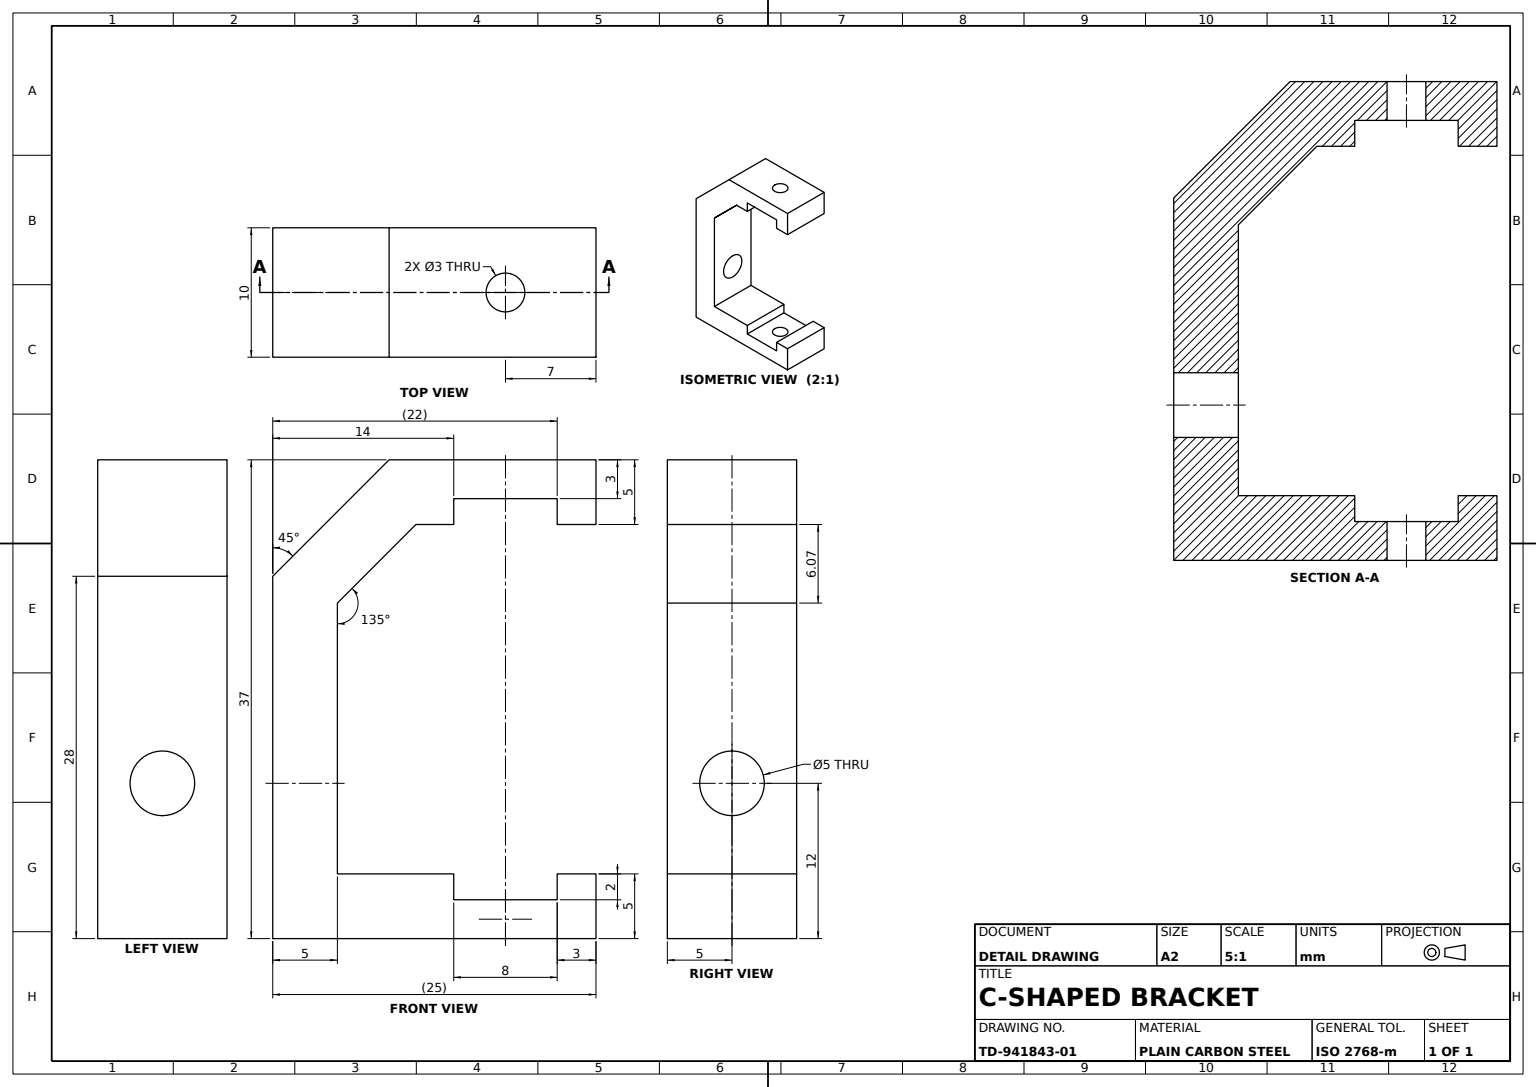
from build123d import *

# Parameters (mm, degrees)
C_BRACKET_BODY_DEPTH = 5
FLANGE_HOLE_SKETCH_R = 1.5
FLANGE_HOLES_3_DEPTH = 100
WEB_HOLE_SKETCH_R    = 2.5
WEB_HOLE_DEPTH       = 100


with BuildPart() as part:
    # C Profile Sketch → C Bracket Body (new, symmetric)
    with BuildSketch(Plane.XY):
        Polygon((0, 0), (0, 28), (9, 37), (25, 37), (25, 32), (22, 32), (22, 34), (14, 34), (14, 32), (11.071067812, 32), (5, 25.928932188), (5, 5), (14, 5), (14, 3), (22, 3), (22, 5), (25, 5), (25, 0), align=None)
    extrude(amount=C_BRACKET_BODY_DEPTH, both=True)

    # Flange Hole Sketch → Flange Holes Ø3 (cut, symmetric)
    with BuildSketch(Plane.XZ.offset(-34)):
        with Locations(Location((18, 0, 0), (0, 0, 270))):
            Circle(FLANGE_HOLE_SKETCH_R)
    extrude(amount=FLANGE_HOLES_3_DEPTH, both=True, mode=Mode.SUBTRACT)

    # Web Hole Sketch → Web Hole (cut, symmetric)
    with BuildSketch(Plane(origin=(5, 0, 0), x_dir=(0, 0, -1), z_dir=(1, 0, 0))):
        with Locations((0, 12)):
            Circle(WEB_HOLE_SKETCH_R)
    extrude(amount=WEB_HOLE_DEPTH, both=True, mode=Mode.SUBTRACT)


solid = part.part
